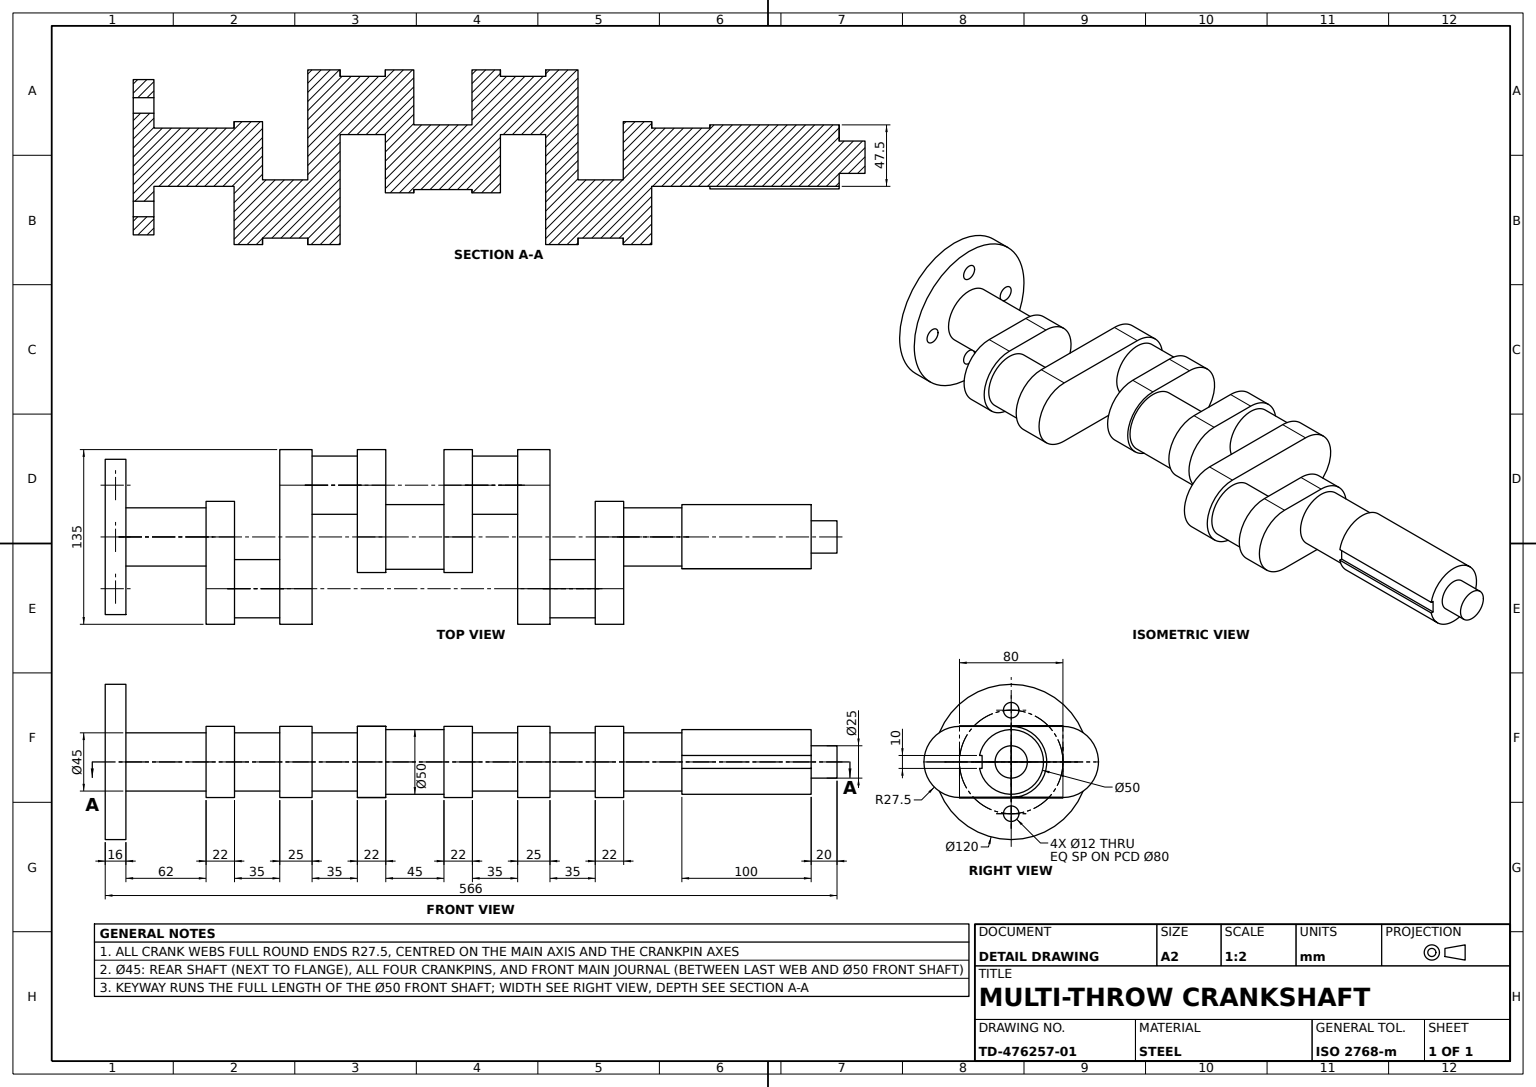
from build123d import *

# Parameters (mm, degrees)
WEB_1_DEPTH                   = 22
CRANKPIN_1_SKETCH_R           = 22.5
CRANKPIN_1_45_DEPTH           = 35
WEB_2_DEPTH                   = 25
CRANKPIN_2_SKETCH_R           = 22.5
CRANKPIN_2_45_DEPTH           = 35
WEB_3_DEPTH                   = 22
CENTRE_MAIN_JOURNAL_SKETCH_R  = 25
CENTRE_MAIN_JOURNAL_50_DEPTH  = 45
WEB_4_DEPTH                   = 22
CRANKPIN_3_SKETCH_R           = 22.5
CRANKPIN_3_45_DEPTH           = 35
WEB_5_DEPTH                   = 25
CRANKPIN_4_SKETCH_R           = 22.5
CRANKPIN_4_45_DEPTH           = 35
WEB_6_DEPTH                   = 22
FRONT_START                   = 45
FRONT_JOURNAL_SKETCH_R        = 22.5
FRONT_JOURNAL_45_DEPTH        = 45
FRONT_SHAFT_SKETCH_R          = 25
FRONT_SHAFT_50_DEPTH          = 100
NOSE_SKETCH_R                 = 12.5
NOSE_25_DEPTH                 = 20
FLANGE_BOLT_HOLES_SKETCH_R    = 6
FLANGE_BOLT_HOLES_4X_12_DEPTH = 20
KEYWAY_SKETCH_W               = 5
KEYWAY_SKETCH_H               = 10
KEYWAY_10X5_DEPTH             = 110


with BuildPart() as part:
    # Flange Profile Sketch → Flange and Rear Shaft (revolve)
    with BuildSketch(Plane.XY, mode=Mode.PRIVATE) as flange_and_rear_shaft_sk:
        Polygon((0, 0), (0, 60), (16, 60), (16, 22.5), (78, 22.5), (78, 0), align=None)
    revolve(flange_and_rear_shaft_sk.sketch.rotate(Axis((-89.086419753, 0, 0), (1, 0, 0)), 90), axis=Axis((-89.086419753, 0, 0), (1, 0, 0)))

    # Web 1 Sketch → Web 1 (add)
    with BuildSketch(Plane(origin=(78, 0, 0), x_dir=(0, 0, -1), z_dir=(1, 0, 0))):
        with BuildLine():
            Line((0, -27.5), (-40, -27.5))
            ThreePointArc((-40, -27.5), (-67.5, 0), (-40, 27.5))
            Line((-40, 27.5), (0, 27.5))
            ThreePointArc((0, 27.5), (27.5, 0), (0, -27.5))
        make_face()
    extrude(amount=WEB_1_DEPTH)

    # Crankpin 1 Sketch → Crankpin 1 Ø45 (add)
    with BuildSketch(Plane(origin=(100, 0, 0), x_dir=(0, 0, -1), z_dir=(1, 0, 0))):
        with Locations((-40, 0)):
            Circle(CRANKPIN_1_SKETCH_R)
    extrude(amount=CRANKPIN_1_45_DEPTH)

    # Web 2 Sketch → Web 2 (add)
    with BuildSketch(Plane(origin=(135, 0, 0), x_dir=(0, 0, -1), z_dir=(1, 0, 0))):
        with BuildLine():
            Line((-40, 27.5), (40, 27.5))
            ThreePointArc((40, 27.5), (67.5, 0), (40, -27.5))
            Line((40, -27.5), (-40, -27.5))
            ThreePointArc((-40, -27.5), (-67.5, 0), (-40, 27.5))
        make_face()
    extrude(amount=WEB_2_DEPTH)

    # Crankpin 2 Sketch → Crankpin 2 Ø45 (add)
    with BuildSketch(Plane(origin=(160, 0, 0), x_dir=(0, 0, -1), z_dir=(1, 0, 0))):
        with Locations((40, 0)):
            Circle(CRANKPIN_2_SKETCH_R)
    extrude(amount=CRANKPIN_2_45_DEPTH)

    # Web 3 Sketch → Web 3 (add)
    with BuildSketch(Plane(origin=(195, 0, 0), x_dir=(0, 0, -1), z_dir=(1, 0, 0))):
        with BuildLine():
            Line((40, -27.5), (0, -27.5))
            ThreePointArc((0, -27.5), (-27.5, 0), (0, 27.5))
            Line((0, 27.5), (40, 27.5))
            ThreePointArc((40, 27.5), (67.5, 0), (40, -27.5))
        make_face()
    extrude(amount=WEB_3_DEPTH)

    # Centre Main Journal Sketch → Centre Main Journal Ø50 (add)
    with BuildSketch(Plane(origin=(217, 0, 0), x_dir=(0, 0, -1), z_dir=(1, 0, 0))):
        with Locations(Location((0, 0, 0), (0, 0, 180))):
            Circle(CENTRE_MAIN_JOURNAL_SKETCH_R)
    extrude(amount=CENTRE_MAIN_JOURNAL_50_DEPTH)

    # Web 4 Sketch → Web 4 (add)
    with BuildSketch(Plane(origin=(262, 0, 0), x_dir=(0, 0, -1), z_dir=(1, 0, 0))):
        with BuildLine():
            Line((0, 27.5), (40, 27.5))
            ThreePointArc((40, 27.5), (67.5, 0), (40, -27.5))
            Line((40, -27.5), (0, -27.5))
            ThreePointArc((0, -27.5), (-27.5, 0), (0, 27.5))
        make_face()
    extrude(amount=WEB_4_DEPTH)

    # Crankpin 3 Sketch → Crankpin 3 Ø45 (add)
    with BuildSketch(Plane(origin=(284, 0, 0), x_dir=(0, 0, -1), z_dir=(1, 0, 0))):
        with Locations((40, 0)):
            Circle(CRANKPIN_3_SKETCH_R)
    extrude(amount=CRANKPIN_3_45_DEPTH)

    # Web 5 Sketch → Web 5 (add)
    with BuildSketch(Plane(origin=(319, 0, 0), x_dir=(0, 0, -1), z_dir=(1, 0, 0))):
        with BuildLine():
            Line((40, -27.5), (-40, -27.5))
            ThreePointArc((-40, -27.5), (-67.5, 0), (-40, 27.5))
            Line((-40, 27.5), (40, 27.5))
            ThreePointArc((40, 27.5), (67.5, 0), (40, -27.5))
        make_face()
    extrude(amount=WEB_5_DEPTH)

    # Crankpin 4 Sketch → Crankpin 4 Ø45 (add)
    with BuildSketch(Plane(origin=(344, 0, 0), x_dir=(0, 0, -1), z_dir=(1, 0, 0))):
        with Locations((-40, 0)):
            Circle(CRANKPIN_4_SKETCH_R)
    extrude(amount=CRANKPIN_4_45_DEPTH)

    # Web 6 Sketch → Web 6 (add)
    with BuildSketch(Plane(origin=(379, 0, 0), x_dir=(0, 0, -1), z_dir=(1, 0, 0))):
        with BuildLine():
            Line((-40, 27.5), (0, 27.5))
            ThreePointArc((0, 27.5), (27.5, 0), (0, -27.5))
            Line((0, -27.5), (-40, -27.5))
            ThreePointArc((-40, -27.5), (-67.5, 0), (-40, 27.5))
        make_face()
    extrude(amount=WEB_6_DEPTH)

    # Front Journal Sketch → Front Journal Ø45 (add)
    with BuildSketch(Plane(origin=(401, 0, 0), x_dir=(0, 0, -1), z_dir=(1, 0, 0)).offset(FRONT_START)):
        with Locations(Location((0, 0, 0), (0, 0, 180))):
            Circle(FRONT_JOURNAL_SKETCH_R)
    extrude(amount=-FRONT_JOURNAL_45_DEPTH)

    # Front Shaft Sketch → Front Shaft Ø50 (add)
    with BuildSketch(Plane(origin=(446, 0, 0), x_dir=(0, 0, -1), z_dir=(1, 0, 0))):
        with Locations(Location((0, 0, 0), (0, 0, 180))):
            Circle(FRONT_SHAFT_SKETCH_R)
    extrude(amount=FRONT_SHAFT_50_DEPTH)

    # Nose Sketch → Nose Ø25 (add)
    with BuildSketch(Plane(origin=(546, 0, 0), x_dir=(0, 0, -1), z_dir=(1, 0, 0))):
        Circle(NOSE_SKETCH_R)
    extrude(amount=NOSE_25_DEPTH)

    # Flange Bolt Holes Sketch → Flange Bolt Holes 4xØ12 (cut)
    with BuildSketch(Plane.ZY):
        with Locations((0, 40)):
            Circle(FLANGE_BOLT_HOLES_SKETCH_R)
        with Locations((40, 0)):
            Circle(FLANGE_BOLT_HOLES_SKETCH_R)
        with Locations((0, -40)):
            Circle(FLANGE_BOLT_HOLES_SKETCH_R)
        with Locations((-40, 0)):
            Circle(FLANGE_BOLT_HOLES_SKETCH_R)
    extrude(amount=-FLANGE_BOLT_HOLES_4X_12_DEPTH, mode=Mode.SUBTRACT)

    # Keyway Sketch → Keyway 10x5 (cut)
    with BuildSketch(Plane(origin=(546, 0, 0), x_dir=(0, 0, -1), z_dir=(1, 0, 0))):
        with Locations((-25, 0)):
            Rectangle(KEYWAY_SKETCH_W, KEYWAY_SKETCH_H)
    extrude(amount=-KEYWAY_10X5_DEPTH, mode=Mode.SUBTRACT)


solid = part.part
